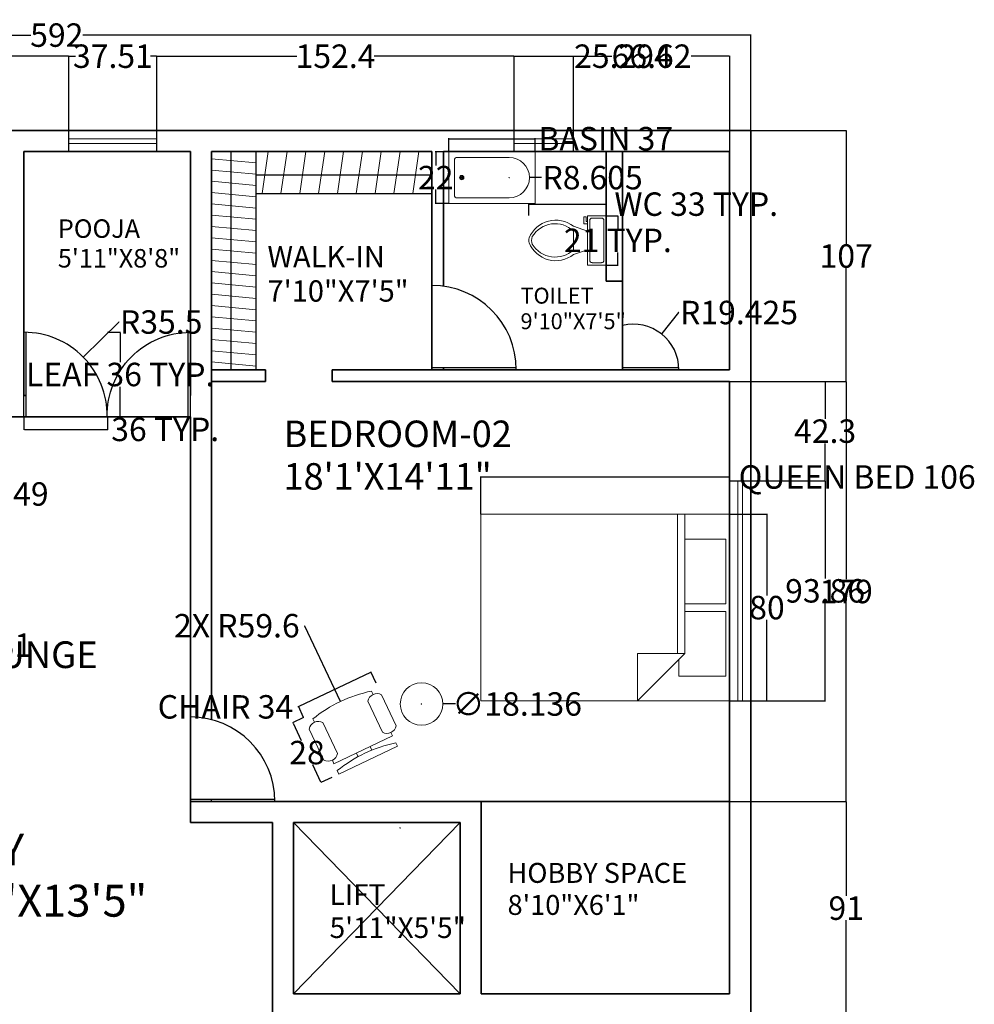
# Model space of a CAD drawing. Units: inches. Extents: x 135 to 880, y 60 to 879.
# Tile 5 of 5: x 473 to 880, y 459 to 879. Entities that reach past the tile are written whole.
import ezdxf

# ---------------------------------------------------------------- set-up
doc = ezdxf.new("R2010")
doc.units = ezdxf.units.IN
doc.header["$MEASUREMENT"] = 0
for name, color, linetype, lineweight in [('A-ANNO-DIMS', 2, 'Continuous', 18), ('A-AREA-IDEN', 7, 'Continuous', 18), ('A-DOOR', 3, 'Continuous', 25), ('A-FLOR-CASE', 32, 'Continuous', 25), ('A-FLOR-CASE-PATT', 252, 'Continuous', 13), ('A-FLOR-FIXT', 9, 'Continuous', 20), ('A-FLOR-OPEN', 8, 'Continuous', 18), ('A-FURN', 8, 'Continuous', 18), ('A-GLAZ', 4, 'Continuous', 18), ('A-WALL', 7, 'Continuous', 35)]:
    doc.layers.add(name, color=color, linetype=linetype, lineweight=lineweight)
doc.styles.get("Standard").update_dxf_attribs({"font": 'arial.ttf'})
doc.dimstyles.get("Standard").update_dxf_attribs({"dimtxt": 10, "dimasz": 0.18, "dimexe": 0.18, "dimexo": 0.0625, "dimgap": 0.09, "dimtad": 0, "dimtih": 1, "dimtoh": 1, "dimdec": 0, "dimzin": 0, "dimdsep": 46, "dimlunit": 3, "dimtxsty": 'Standard', "dimcen": 0.09, "dimadec": 0, "dimazin": 0, "dimtfac": 1, "dimtdec": 0, "dimtofl": 0, "dimtmove": 0, "dimatfit": 3, "dimfxl": 1, "dimtolj": 1, "dimtzin": 0, "dimarcsym": 0})

# ---------------------------------------------------------------- blocks, each defined once
blk = doc.blocks.new('Toilet - top')
for p, q in [((9.5, -6), (9.5, -2)), ((-8, -8.5), (-8, -8)), ((-7, -8), (-7, -9.5)), ((-4, -8), (-6, -14)), ((4, -8), (6, -14)), ((-10, -8.5), (-8, -8.5)), ((-10, -9.5), (-10, -8.5)), ((-7, -9.5), (-10, -9.5)), ((4, -14), (-4, -14))]:
    blk.add_line(p, q)
blk.add_lwpolyline([(10.5, -8), (10.5, 0), (-10.5, 0), (-10.5, -8)], close=True)
for points in [[(-9.5, -2), (-9.5, -6)], [(8.5, -1), (-8.5, -1)], [(-8.5, -7), (8.5, -7)]]:
    blk.add_lwpolyline(points)
for centre, radius, start, end in [((-8.62, -1.88), 0.884, 81.8699, 188.1301), ((8.62, -1.88), 0.884, 351.8699, 98.1301), ((-8.62, -6.12), 0.884, 171.8699, 278.1301), ((8.62, -6.12), 0.884, 261.8699, 8.1301), ((3.52, -21.58), 12.17, 141.4691, 247.9714), ((4.2, -21.82), 11.33, 136.3677, 238.9468), ((-3.52, -21.58), 12.17, 292.0284, 38.5307), ((-4.2, -21.82), 11.33, 301.053, 43.6321), ((0, -27.88), 4, 245.7318, 294.2682), ((0, -29), 4, 254.8605, 285.1395)]:
    blk.add_arc(centre, radius, start, end)
blk = doc.blocks.new('Bath Tub - 26 x 60 in.')
for p, q in [((8, -18), (10, -18)), ((9, -17), (9, -19))]:
    blk.add_line(p, q)
blk.add_lwpolyline([(0, -36), (0, 0), (60, 0), (60, -36)], close=True)
for points in [[(4, -30), (4, -6)], [(6, -4), (42, -4)], [(42, -32), (6, -32)]]:
    blk.add_lwpolyline(points)
for radius in [1.5, 1]:
    blk.add_circle((9, -18), radius)
for centre, radius, start, end in [((5.75, -5.75), 1.77, 81.8699, 188.1301), ((42, -18), 14, 270, 90), ((5.75, -30.25), 1.77, 171.8699, 278.1301)]:
    blk.add_arc(centre, radius, start, end)
blk = doc.blocks.new('Bed - Queen')
for p, q in [((0, -80.00003), (0, 0)), ((0, 0), (59.99999, 0)), ((59.99999, 0), (59.99999, -80.00003)), ((7.99999, -1.2), (28.79998, -1.2)), ((7.99999, -14.4), (7.99999, -1.2)), ((28.79998, -1.2), (28.79998, -14.4)), ((31.19999, -1.2), (51.99999, -1.2)), ((31.19999, -14.4), (31.19999, -1.2)), ((51.99999, -1.2), (51.99999, -16.4)), ((0, -14.4), (44.8, -14.4)), ((59.99999, -29.6), (44.8, -14.4)), ((44.8, -14.4), (44.8, -29.6)), ((44.8, -16.8), (0, -16.8)), ((51.99999, -16.4), (46.79936, -16.4)), ((44.8, -29.6), (59.99999, -29.6)), ((59.99999, -80.00003), (0, -80.00003))]:
    blk.add_line(p, q)
blk = doc.blocks.new('Chair - Desk')
for p, q in [((-8.5, 0), (-8.5, -1)), ((-8.5, 0), (8.5, 0)), ((8.5, 0), (8.5, -1)), ((-2, -3), (-2, -1.9355)), ((2, -1.9576), (2, -3)), ((-10.5, -5), (-10.5, -14)), ((-8.5, -3), (-8.5, -4)), ((-8.5, -3), (8.5, -3)), ((-6.5, -14), (-6.5, -5)), ((6.5, -5), (6.5, -14)), ((8.5, -3), (8.5, -4)), ((10.5, -14), (10.5, -5)), ((-8.5, -15), (-8.5, -16)), ((8.5, -15), (8.5, -16))]:
    blk.add_line(p, q)
for centre, radius, start, end in [((0, 34.625), 36.625, 256.5803, 283.4197), ((-8.5, -6.5), 2.5, 36.8699, 143.1301), ((8.5, -6.5), 2.5, 36.8699, 143.1301), ((-8.5, -12.5), 2.5, 216.8699, 323.1301), ((8.5, -12.5), 2.5, 216.8699, 323.1301), ((0, 19.625), 36.625, 256.5803, 283.4197)]:
    blk.add_arc(centre, radius, start, end)
blk = doc.blocks.new('DOOR-SWING-36IN')
for p, q in [((36, 36), (0, 36)), ((36, 35), (0, 35))]:
    blk.add_line(p, q)
blk.add_arc((36, 36), 36, 180, 270)
blk = doc.blocks.new('DOOR-PAIRED-LEAF-36IN')
for p, q in [((0, 0), (0, 36)), ((1, 0), (1, 36))]:
    blk.add_line(p, q)
blk.add_arc((0, 0.5), 35.5, 359.1987, 90)
blk = doc.blocks.new('*D12')
at = {"layer": 'A-ANNO-DIMS', "color": 0, "lineweight": -2, "transparency": 16777216}
for p, q in [((402.69, 638.57), (399.13, 635.46)), ((399.38, 635.45), (419.31, 612.59)), ((422.85, 615.44), (419.29, 612.34)), ((419.42, 612.45), (419.54, 612.32)), ((419.54, 612.32), (419.72, 612.32))]:
    blk.add_line(p, q, dxfattribs=at)
at = {"layer": 'A-ANNO-DIMS', "color": 0, "transparency": 16777216}
for points in [[(399.41, 635.47), (399.36, 635.43), (399.27, 635.58)], [(419.33, 612.61), (419.28, 612.57), (419.42, 612.45)]]:
    blk.add_solid(points, dxfattribs=at)
at = {"layer": 'Defpoints', "color": 0, "transparency": 16777216}
for p in [(402.73, 638.61), (422.89, 615.48), (419.42, 612.45)]:
    blk.add_point(p, dxfattribs=at)
at = {"layer": 'A-ANNO-DIMS', "color": 0, "transparency": 16777216, "insert": (449.62, 612.32), "char_height": 10, "attachment_point": 5}
blk.add_mtext('\\A1;CHAIR 31', dxfattribs=at)
blk = doc.blocks.new('*D16')
at = {"layer": 'A-ANNO-DIMS', "color": 0, "lineweight": -2, "transparency": 16777216}
for p, q in [((622.81, 600.64), (592.25, 586.17)), ((625.14, 596.14), (622.89, 600.88)), ((591.93, 586.01), (591.75, 586.01)), ((592.09, 586.09), (591.93, 586.01)), ((594.26, 581.51), (592.01, 586.25))]:
    blk.add_line(p, q, dxfattribs=at)
at = {"layer": 'A-ANNO-DIMS', "color": 0, "transparency": 16777216}
for points in [[(622.8, 600.67), (622.82, 600.61), (622.97, 600.72)], [(592.24, 586.19), (592.26, 586.14), (592.09, 586.09)]]:
    blk.add_solid(points, dxfattribs=at)
at = {"layer": 'Defpoints', "color": 0, "transparency": 16777216}
for p in [(625.17, 596.09), (592.09, 586.09), (594.28, 581.46)]:
    blk.add_point(p, dxfattribs=at)
at = {"layer": 'A-ANNO-DIMS', "color": 0, "transparency": 16777216, "insert": (560.9, 586.01), "char_height": 10, "attachment_point": 5}
blk.add_mtext('\\A1;CHAIR 34', dxfattribs=at)
blk = doc.blocks.new('*D17')
at = {"layer": 'A-ANNO-DIMS', "color": 0, "lineweight": -2, "transparency": 16777216}
for p, q in [((594.23, 581.43), (589.49, 579.19)), ((589.73, 579.1), (593.23, 571.71)), ((601.65, 553.94), (598.15, 561.32)), ((606.3, 555.94), (601.56, 553.7))]:
    blk.add_line(p, q, dxfattribs=at)
at = {"layer": 'A-ANNO-DIMS', "color": 0, "transparency": 16777216}
for points in [[(589.76, 579.11), (589.7, 579.09), (589.65, 579.26)], [(601.68, 553.95), (601.62, 553.92), (601.73, 553.77)]]:
    blk.add_solid(points, dxfattribs=at)
at = {"layer": 'Defpoints', "color": 0, "transparency": 16777216}
for p in [(594.28, 581.46), (606.36, 555.97), (601.73, 553.77)]:
    blk.add_point(p, dxfattribs=at)
at = {"layer": 'A-ANNO-DIMS', "color": 0, "transparency": 16777216, "insert": (595.69, 566.52), "char_height": 10, "attachment_point": 5}
blk.add_mtext('\\A1;28', dxfattribs=at)
blk = doc.blocks.new('*D20')
at = {"layer": 'A-ANNO-DIMS', "color": 0, "lineweight": -2, "transparency": 16777216}
for p, q in [((656.14, 822.76), (656.14, 828.41)), ((656.32, 828.23), (692.84, 828.23)), ((693.02, 822.76), (693.02, 828.41)), ((693.02, 828.23), (693.2, 828.23))]:
    blk.add_line(p, q, dxfattribs=at)
at = {"layer": 'A-ANNO-DIMS', "color": 0, "transparency": 16777216}
for points in [[(656.32, 828.26), (656.32, 828.2), (656.14, 828.23)], [(692.84, 828.26), (692.84, 828.2), (693.02, 828.23)]]:
    blk.add_solid(points, dxfattribs=at)
at = {"layer": 'Defpoints', "color": 0, "transparency": 16777216}
for p in [(693.02, 828.23), (656.14, 822.7), (693.02, 822.7)]:
    blk.add_point(p, dxfattribs=at)
at = {"layer": 'A-ANNO-DIMS', "color": 0, "transparency": 16777216, "insert": (723.13, 828.23), "char_height": 10, "attachment_point": 5}
blk.add_mtext('\\A1;BASIN 37', dxfattribs=at)
blk = doc.blocks.new('*D21')
at = {"layer": 'A-ANNO-DIMS', "color": 0, "lineweight": -2, "transparency": 16777216}
for p, q in [((656.08, 822.7), (650.43, 822.7)), ((650.61, 822.52), (650.61, 816.75)), ((650.61, 800.75), (650.61, 806.53)), ((656.08, 800.57), (650.43, 800.57))]:
    blk.add_line(p, q, dxfattribs=at)
at = {"layer": 'A-ANNO-DIMS', "color": 0, "transparency": 16777216}
for points in [[(650.58, 822.52), (650.64, 822.52), (650.61, 822.7)], [(650.58, 800.75), (650.64, 800.75), (650.61, 800.57)]]:
    blk.add_solid(points, dxfattribs=at)
at = {"layer": 'Defpoints', "color": 0, "transparency": 16777216}
for p in [(650.61, 822.7), (656.14, 822.7), (656.14, 800.57)]:
    blk.add_point(p, dxfattribs=at)
at = {"layer": 'A-ANNO-DIMS', "color": 0, "transparency": 16777216, "insert": (650.61, 811.64), "char_height": 10, "attachment_point": 5}
blk.add_mtext('\\A1;22', dxfattribs=at)
blk = doc.blocks.new('*D28')
at = {"layer": 'A-ANNO-DIMS', "color": 0, "lineweight": -2, "transparency": 16777216}
for p, q in [((669.88, 668.17), (669.88, 684.2)), ((670.06, 684.02), (775.8, 684.02)), ((775.98, 668.17), (775.98, 684.2)), ((775.98, 684.02), (776.16, 684.02))]:
    blk.add_line(p, q, dxfattribs=at)
at = {"layer": 'A-ANNO-DIMS', "color": 0, "transparency": 16777216}
for points in [[(670.06, 684.05), (670.06, 683.99), (669.88, 684.02)], [(775.8, 684.05), (775.8, 683.99), (775.98, 684.02)]]:
    blk.add_solid(points, dxfattribs=at)
at = {"layer": 'Defpoints', "color": 0, "transparency": 16777216}
for p in [(775.98, 684.02), (669.88, 668.1), (775.98, 668.1)]:
    blk.add_point(p, dxfattribs=at)
at = {"layer": 'A-ANNO-DIMS', "color": 0, "transparency": 16777216, "insert": (830.36, 684.02), "char_height": 10, "attachment_point": 5}
blk.add_mtext('\\A1;QUEEN BED 106', dxfattribs=at)
blk = doc.blocks.new('*D29')
at = {"layer": 'A-ANNO-DIMS', "color": 0, "lineweight": -2, "transparency": 16777216}
for p, q in [((776.04, 668.1), (792.07, 668.1)), ((791.89, 667.92), (791.89, 633.52)), ((791.89, 588.72), (791.89, 623.12)), ((776.04, 588.54), (792.07, 588.54))]:
    blk.add_line(p, q, dxfattribs=at)
at = {"layer": 'A-ANNO-DIMS', "color": 0, "transparency": 16777216}
for points in [[(791.86, 667.92), (791.92, 667.92), (791.89, 668.1)], [(791.86, 588.72), (791.92, 588.72), (791.89, 588.54)]]:
    blk.add_solid(points, dxfattribs=at)
at = {"layer": 'Defpoints', "color": 0, "transparency": 16777216}
for p in [(775.98, 668.1), (775.98, 588.54), (791.89, 588.54)]:
    blk.add_point(p, dxfattribs=at)
at = {"layer": 'A-ANNO-DIMS', "color": 0, "transparency": 16777216, "insert": (791.89, 628.32), "char_height": 10, "attachment_point": 5}
blk.add_mtext('\\A1;80', dxfattribs=at)
blk = doc.blocks.new('*D30')
at = {"layer": 'A-ANNO-DIMS', "color": 0, "lineweight": -2, "transparency": 16777216}
for p, q in [((690.28, 795.44), (690.28, 800.51)), ((690.46, 800.33), (723.15, 800.33)), ((723.33, 795.44), (723.33, 800.51)), ((723.33, 800.33), (723.51, 800.33))]:
    blk.add_line(p, q, dxfattribs=at)
at = {"layer": 'A-ANNO-DIMS', "color": 0, "transparency": 16777216}
for points in [[(690.46, 800.36), (690.46, 800.3), (690.28, 800.33)], [(723.15, 800.36), (723.15, 800.3), (723.33, 800.33)]]:
    blk.add_solid(points, dxfattribs=at)
at = {"layer": 'Defpoints', "color": 0, "transparency": 16777216}
for p in [(723.33, 800.33), (690.28, 795.38), (723.33, 795.38)]:
    blk.add_point(p, dxfattribs=at)
at = {"layer": 'A-ANNO-DIMS', "color": 0, "transparency": 16777216, "insert": (761.72, 800.33), "char_height": 10, "attachment_point": 5}
blk.add_mtext('\\A1;WC 33 TYP.', dxfattribs=at)
blk = doc.blocks.new('*D31')
at = {"layer": 'A-ANNO-DIMS', "color": 0, "lineweight": -2, "transparency": 16777216}
for p, q in [((723.39, 795.38), (728.47, 795.38)), ((728.29, 795.2), (728.29, 789.99)), ((728.29, 774.56), (728.29, 779.76)), ((723.39, 774.38), (728.47, 774.38))]:
    blk.add_line(p, q, dxfattribs=at)
at = {"layer": 'A-ANNO-DIMS', "color": 0, "transparency": 16777216}
for points in [[(728.26, 795.2), (728.32, 795.2), (728.29, 795.38)], [(728.26, 774.56), (728.32, 774.56), (728.29, 774.38)]]:
    blk.add_solid(points, dxfattribs=at)
at = {"layer": 'Defpoints', "color": 0, "transparency": 16777216}
for p in [(723.33, 795.38), (723.33, 774.38), (728.29, 774.38)]:
    blk.add_point(p, dxfattribs=at)
at = {"layer": 'A-ANNO-DIMS', "color": 0, "transparency": 16777216, "insert": (728.29, 784.88), "char_height": 10, "attachment_point": 5}
blk.add_mtext('\\A1;21 TYP.', dxfattribs=at)
blk = doc.blocks.new('*D34')
at = {"layer": 'A-ANNO-DIMS', "color": 0, "lineweight": -2, "transparency": 16777216}
for p, q in [((510.67, 745.7), (516.19, 745.7)), ((516.01, 745.52), (516.01, 732.9)), ((516.01, 709.88), (516.01, 722.5)), ((510.67, 709.7), (516.19, 709.7))]:
    blk.add_line(p, q, dxfattribs=at)
at = {"layer": 'A-ANNO-DIMS', "color": 0, "transparency": 16777216}
for points in [[(515.98, 745.52), (516.04, 745.52), (516.01, 745.7)], [(515.98, 709.88), (516.04, 709.88), (516.01, 709.7)]]:
    blk.add_solid(points, dxfattribs=at)
at = {"layer": 'Defpoints', "color": 0, "transparency": 16777216}
for p in [(510.61, 745.7), (516.01, 745.7), (510.61, 709.7)]:
    blk.add_point(p, dxfattribs=at)
at = {"layer": 'A-ANNO-DIMS', "color": 0, "transparency": 16777216, "insert": (516.01, 727.7), "char_height": 10, "attachment_point": 5}
blk.add_mtext('\\A1;LEAF 36 TYP.', dxfattribs=at)
blk = doc.blocks.new('*D35')
at = {"layer": 'A-ANNO-DIMS', "color": 0, "lineweight": -2, "transparency": 16777216}
for p, q in [((474.98, 709.64), (474.98, 704.12)), ((510.61, 709.64), (510.61, 704.12)), ((475.16, 704.3), (510.43, 704.3)), ((510.61, 704.3), (510.79, 704.3))]:
    blk.add_line(p, q, dxfattribs=at)
at = {"layer": 'A-ANNO-DIMS', "color": 0, "transparency": 16777216}
for points in [[(475.16, 704.33), (475.16, 704.27), (474.98, 704.3)], [(510.43, 704.33), (510.43, 704.27), (510.61, 704.3)]]:
    blk.add_solid(points, dxfattribs=at)
at = {"layer": 'Defpoints', "color": 0, "transparency": 16777216}
for p in [(474.98, 709.7), (510.61, 709.7), (510.61, 704.3)]:
    blk.add_point(p, dxfattribs=at)
at = {"layer": 'A-ANNO-DIMS', "color": 0, "transparency": 16777216, "insert": (535.21, 704.3), "char_height": 10, "attachment_point": 5}
blk.add_mtext('\\A1;36 TYP.', dxfattribs=at)
blk = doc.blocks.new('*D38')
at = {"layer": 'A-ANNO-DIMS', "color": 0, "lineweight": -2, "transparency": 16777216}
for p, q in [((192.98, 831.76), (192.98, 872.58)), ((193.16, 872.4), (477.89, 872.4)), ((784.8, 872.4), (500.06, 872.4)), ((784.98, 831.76), (784.98, 872.58))]:
    blk.add_line(p, q, dxfattribs=at)
at = {"layer": 'A-ANNO-DIMS', "color": 0, "transparency": 16777216}
for points in [[(193.16, 872.43), (193.16, 872.37), (192.98, 872.4)], [(784.8, 872.43), (784.8, 872.37), (784.98, 872.4)]]:
    blk.add_solid(points, dxfattribs=at)
at = {"layer": 'Defpoints', "color": 0, "transparency": 16777216}
for p in [(784.98, 872.4), (192.98, 831.7), (784.98, 831.7)]:
    blk.add_point(p, dxfattribs=at)
at = {"layer": 'A-ANNO-DIMS', "color": 0, "transparency": 16777216, "insert": (488.98, 872.4), "char_height": 10, "attachment_point": 5}
blk.add_mtext('\\A1;592', dxfattribs=at)
blk = doc.blocks.new('*D40')
at = {"layer": 'A-ANNO-DIMS', "color": 0, "lineweight": -2, "transparency": 16777216}
for p, q in [((192.98, 822.76), (192.98, 863.58)), ((193.16, 863.4), (326.65, 863.4)), ((493.97, 863.4), (360.47, 863.4)), ((494.15, 822.76), (494.15, 863.58))]:
    blk.add_line(p, q, dxfattribs=at)
at = {"layer": 'A-ANNO-DIMS', "color": 0, "transparency": 16777216}
for points in [[(193.16, 863.43), (193.16, 863.37), (192.98, 863.4)], [(493.97, 863.43), (493.97, 863.37), (494.15, 863.4)]]:
    blk.add_solid(points, dxfattribs=at)
at = {"layer": 'Defpoints', "color": 0, "transparency": 16777216}
for p in [(494.15, 863.4), (192.98, 822.7), (494.15, 822.7)]:
    blk.add_point(p, dxfattribs=at)
at = {"layer": 'A-ANNO-DIMS', "color": 0, "transparency": 16777216, "insert": (343.56, 863.4), "char_height": 10, "attachment_point": 5}
blk.add_mtext('\\A1;301.2', dxfattribs=at)
blk = doc.blocks.new('*D41')
at = {"layer": 'A-ANNO-DIMS', "color": 0, "lineweight": -2, "transparency": 16777216}
for p, q in [((494.15, 822.76), (494.15, 863.58)), ((494.33, 863.4), (496.91, 863.4)), ((531.47, 863.4), (528.89, 863.4)), ((531.65, 822.76), (531.65, 863.58))]:
    blk.add_line(p, q, dxfattribs=at)
at = {"layer": 'A-ANNO-DIMS', "color": 0, "transparency": 16777216}
for points in [[(494.33, 863.43), (494.33, 863.37), (494.15, 863.4)], [(531.47, 863.43), (531.47, 863.37), (531.65, 863.4)]]:
    blk.add_solid(points, dxfattribs=at)
at = {"layer": 'Defpoints', "color": 0, "transparency": 16777216}
for p in [(531.65, 863.4), (494.15, 822.7), (531.65, 822.7)]:
    blk.add_point(p, dxfattribs=at)
at = {"layer": 'A-ANNO-DIMS', "color": 0, "transparency": 16777216, "insert": (512.9, 863.4), "char_height": 10, "attachment_point": 5}
blk.add_mtext('\\A1;37.51', dxfattribs=at)
blk = doc.blocks.new('*D42')
at = {"layer": 'A-ANNO-DIMS', "color": 0, "lineweight": -2, "transparency": 16777216}
for p, q in [((531.65, 822.76), (531.65, 863.58)), ((531.83, 863.4), (591.38, 863.4)), ((683.88, 863.4), (624.33, 863.4)), ((684.06, 822.76), (684.06, 863.58))]:
    blk.add_line(p, q, dxfattribs=at)
at = {"layer": 'A-ANNO-DIMS', "color": 0, "transparency": 16777216}
for points in [[(531.83, 863.43), (531.83, 863.37), (531.65, 863.4)], [(683.88, 863.43), (683.88, 863.37), (684.06, 863.4)]]:
    blk.add_solid(points, dxfattribs=at)
at = {"layer": 'Defpoints', "color": 0, "transparency": 16777216}
for p in [(684.06, 863.4), (531.65, 822.7), (684.06, 822.7)]:
    blk.add_point(p, dxfattribs=at)
at = {"layer": 'A-ANNO-DIMS', "color": 0, "transparency": 16777216, "insert": (607.86, 863.4), "char_height": 10, "attachment_point": 5}
blk.add_mtext('\\A1;152.4', dxfattribs=at)
blk = doc.blocks.new('*D43')
at = {"layer": 'A-ANNO-DIMS', "color": 0, "lineweight": -2, "transparency": 16777216}
for p, q in [((684.06, 822.76), (684.06, 863.58)), ((684.24, 863.4), (709.17, 863.4)), ((709.35, 822.76), (709.35, 863.58)), ((709.35, 863.4), (709.53, 863.4))]:
    blk.add_line(p, q, dxfattribs=at)
at = {"layer": 'A-ANNO-DIMS', "color": 0, "transparency": 16777216}
for points in [[(684.24, 863.43), (684.24, 863.37), (684.06, 863.4)], [(709.17, 863.43), (709.17, 863.37), (709.35, 863.4)]]:
    blk.add_solid(points, dxfattribs=at)
at = {"layer": 'Defpoints', "color": 0, "transparency": 16777216}
for p in [(709.35, 863.4), (684.06, 822.7), (709.35, 822.7)]:
    blk.add_point(p, dxfattribs=at)
at = {"layer": 'A-ANNO-DIMS', "color": 0, "transparency": 16777216, "insert": (730.44, 863.4), "char_height": 10, "attachment_point": 5}
blk.add_mtext('\\A1;25.294', dxfattribs=at)
blk = doc.blocks.new('*D44')
at = {"layer": 'A-ANNO-DIMS', "color": 0, "lineweight": -2, "transparency": 16777216}
for p, q in [((709.35, 822.76), (709.35, 863.58)), ((709.53, 863.4), (725.73, 863.4)), ((775.8, 863.4), (759.6, 863.4)), ((775.98, 822.76), (775.98, 863.58))]:
    blk.add_line(p, q, dxfattribs=at)
at = {"layer": 'A-ANNO-DIMS', "color": 0, "transparency": 16777216}
for points in [[(709.53, 863.43), (709.53, 863.37), (709.35, 863.4)], [(775.8, 863.43), (775.8, 863.37), (775.98, 863.4)]]:
    blk.add_solid(points, dxfattribs=at)
at = {"layer": 'Defpoints', "color": 0, "transparency": 16777216}
for p in [(775.98, 863.4), (709.35, 822.7), (775.98, 822.7)]:
    blk.add_point(p, dxfattribs=at)
at = {"layer": 'A-ANNO-DIMS', "color": 0, "transparency": 16777216, "insert": (742.66, 863.4), "char_height": 10, "attachment_point": 5}
blk.add_mtext('\\A1;66.62', dxfattribs=at)
blk = doc.blocks.new('*D63')
at = {"layer": 'A-ANNO-DIMS', "color": 0, "lineweight": -2, "transparency": 16777216}
for p, q in [((776.04, 545.7), (825.86, 545.7)), ((825.68, 545.52), (825.68, 505.4)), ((825.68, 454.88), (825.68, 495.01)), ((785.04, 454.7), (825.86, 454.7))]:
    blk.add_line(p, q, dxfattribs=at)
at = {"layer": 'A-ANNO-DIMS', "color": 0, "transparency": 16777216}
for points in [[(825.65, 545.52), (825.71, 545.52), (825.68, 545.7)], [(825.65, 454.88), (825.71, 454.88), (825.68, 454.7)]]:
    blk.add_solid(points, dxfattribs=at)
at = {"layer": 'Defpoints', "color": 0, "transparency": 16777216}
for p in [(775.98, 545.7), (825.68, 545.7), (784.98, 454.7)]:
    blk.add_point(p, dxfattribs=at)
at = {"layer": 'A-ANNO-DIMS', "color": 0, "transparency": 16777216, "insert": (825.68, 500.2), "char_height": 10, "attachment_point": 5}
blk.add_mtext('\\A1;91', dxfattribs=at)
blk = doc.blocks.new('*D64')
at = {"layer": 'A-ANNO-DIMS', "color": 0, "lineweight": -2, "transparency": 16777216}
for p, q in [((776.04, 724.7), (825.86, 724.7)), ((825.68, 724.52), (825.68, 640.4)), ((825.68, 545.88), (825.68, 630.01)), ((776.04, 545.7), (825.86, 545.7))]:
    blk.add_line(p, q, dxfattribs=at)
at = {"layer": 'A-ANNO-DIMS', "color": 0, "transparency": 16777216}
for points in [[(825.65, 724.52), (825.71, 724.52), (825.68, 724.7)], [(825.65, 545.88), (825.71, 545.88), (825.68, 545.7)]]:
    blk.add_solid(points, dxfattribs=at)
at = {"layer": 'Defpoints', "color": 0, "transparency": 16777216}
for p in [(775.98, 724.7), (825.68, 724.7), (775.98, 545.7)]:
    blk.add_point(p, dxfattribs=at)
at = {"layer": 'A-ANNO-DIMS', "color": 0, "transparency": 16777216, "insert": (825.68, 635.2), "char_height": 10, "attachment_point": 5}
blk.add_mtext('\\A1;179', dxfattribs=at)
blk = doc.blocks.new('*D65')
at = {"layer": 'A-ANNO-DIMS', "color": 0, "lineweight": -2, "transparency": 16777216}
for p, q in [((785.04, 831.7), (825.86, 831.7)), ((825.68, 831.52), (825.68, 783.4)), ((825.68, 724.88), (825.68, 773.01)), ((776.04, 724.7), (825.86, 724.7))]:
    blk.add_line(p, q, dxfattribs=at)
at = {"layer": 'A-ANNO-DIMS', "color": 0, "transparency": 16777216}
for points in [[(825.65, 831.52), (825.71, 831.52), (825.68, 831.7)], [(825.65, 724.88), (825.71, 724.88), (825.68, 724.7)]]:
    blk.add_solid(points, dxfattribs=at)
at = {"layer": 'Defpoints', "color": 0, "transparency": 16777216}
for p in [(784.98, 831.7), (825.68, 831.7), (775.98, 724.7)]:
    blk.add_point(p, dxfattribs=at)
at = {"layer": 'A-ANNO-DIMS', "color": 0, "transparency": 16777216, "insert": (825.68, 778.2), "char_height": 10, "attachment_point": 5}
blk.add_mtext('\\A1;107', dxfattribs=at)
blk = doc.blocks.new('*D70')
at = {"layer": 'A-ANNO-DIMS', "color": 0, "lineweight": -2, "transparency": 16777216}
for p, q in [((776.04, 724.7), (816.86, 724.7)), ((816.68, 724.52), (816.68, 708.75)), ((816.68, 682.58), (816.68, 698.35)), ((776.04, 682.4), (816.86, 682.4))]:
    blk.add_line(p, q, dxfattribs=at)
at = {"layer": 'A-ANNO-DIMS', "color": 0, "transparency": 16777216}
for points in [[(816.65, 724.52), (816.71, 724.52), (816.68, 724.7)], [(816.65, 682.58), (816.71, 682.58), (816.68, 682.4)]]:
    blk.add_solid(points, dxfattribs=at)
at = {"layer": 'Defpoints', "color": 0, "transparency": 16777216}
for p in [(775.98, 724.7), (775.98, 682.4), (816.68, 682.4)]:
    blk.add_point(p, dxfattribs=at)
at = {"layer": 'A-ANNO-DIMS', "color": 0, "transparency": 16777216, "insert": (816.68, 703.55), "char_height": 10, "attachment_point": 5}
blk.add_mtext('\\A1;42.3', dxfattribs=at)
blk = doc.blocks.new('*D71')
at = {"layer": 'A-ANNO-DIMS', "color": 0, "lineweight": -2, "transparency": 16777216}
for p, q in [((776.04, 682.4), (816.86, 682.4)), ((816.68, 682.22), (816.68, 640.67)), ((816.68, 588.72), (816.68, 630.27)), ((776.04, 588.54), (816.86, 588.54))]:
    blk.add_line(p, q, dxfattribs=at)
at = {"layer": 'A-ANNO-DIMS', "color": 0, "transparency": 16777216}
for points in [[(816.65, 682.22), (816.71, 682.22), (816.68, 682.4)], [(816.65, 588.72), (816.71, 588.72), (816.68, 588.54)]]:
    blk.add_solid(points, dxfattribs=at)
at = {"layer": 'Defpoints', "color": 0, "transparency": 16777216}
for p in [(775.98, 682.4), (775.98, 588.54), (816.68, 588.54)]:
    blk.add_point(p, dxfattribs=at)
at = {"layer": 'A-ANNO-DIMS', "color": 0, "transparency": 16777216, "insert": (816.68, 635.47), "char_height": 10, "attachment_point": 5}
blk.add_mtext('\\A1;93.86', dxfattribs=at)
blk = doc.blocks.new('*D76')
at = {"layer": 'A-ANNO-DIMS', "color": 0, "lineweight": -2, "transparency": 16777216}
for p, q in [((754.12, 754.13), (747.03, 745.11)), ((754.3, 754.13), (754.12, 754.13)), ((734.82, 729.7), (735, 729.7)), ((734.91, 729.61), (734.91, 729.79))]:
    blk.add_line(p, q, dxfattribs=at)
at = {"layer": 'A-ANNO-DIMS', "color": 0, "transparency": 16777216}
blk.add_solid([(747, 745.13), (747.05, 745.09), (746.91, 744.97)], dxfattribs=at)
at = {"layer": 'Defpoints', "color": 0, "transparency": 16777216}
for p in [(746.91, 744.97), (734.91, 729.7)]:
    blk.add_point(p, dxfattribs=at)
at = {"layer": 'A-ANNO-DIMS', "color": 0, "transparency": 16777216, "insert": (779.97, 754.13), "char_height": 10, "attachment_point": 5}
blk.add_mtext('\\A1;R19.425', dxfattribs=at)
blk = doc.blocks.new('*D77')
at = {"layer": 'A-ANNO-DIMS', "color": 0, "lineweight": -2, "transparency": 16777216}
for p, q in [((515.42, 750.08), (500.38, 735.25)), ((515.6, 750.08), (515.42, 750.08)), ((474.89, 710.2), (475.07, 710.2)), ((474.98, 710.11), (474.98, 710.29))]:
    blk.add_line(p, q, dxfattribs=at)
at = {"layer": 'A-ANNO-DIMS', "color": 0, "transparency": 16777216}
blk.add_solid([(500.36, 735.27), (500.4, 735.23), (500.26, 735.13)], dxfattribs=at)
at = {"layer": 'Defpoints', "color": 0, "transparency": 16777216}
for p in [(500.26, 735.13), (474.98, 710.2)]:
    blk.add_point(p, dxfattribs=at)
at = {"layer": 'A-ANNO-DIMS', "color": 0, "transparency": 16777216, "insert": (533.5, 750.08), "char_height": 10, "attachment_point": 5}
blk.add_mtext('\\A1;R35.5', dxfattribs=at)
blk = doc.blocks.new('*D81')
at = {"layer": 'A-ANNO-DIMS', "color": 0, "lineweight": -2, "transparency": 16777216}
for p, q in [((417.13, 676.77), (417.31, 676.77)), ((417.22, 676.68), (417.22, 676.86)), ((439.22, 676.77), (431.15, 676.77))]:
    blk.add_line(p, q, dxfattribs=at)
at = {"layer": 'A-ANNO-DIMS', "color": 0, "transparency": 16777216}
blk.add_solid([(431.15, 676.8), (431.15, 676.74), (430.97, 676.77)], dxfattribs=at)
at = {"layer": 'Defpoints', "color": 0, "transparency": 16777216}
for p in [(403.48, 676.77), (430.97, 676.77)]:
    blk.add_point(p, dxfattribs=at)
at = {"layer": 'A-ANNO-DIMS', "color": 0, "transparency": 16777216, "insert": (461.63, 676.77), "char_height": 10, "attachment_point": 5}
blk.add_mtext('\\A1;∅27.49', dxfattribs=at)
blk = doc.blocks.new('*D82')
at = {"layer": 'A-ANNO-DIMS', "color": 0, "lineweight": -2, "transparency": 16777216}
for p, q in [((644.45, 587.23), (644.63, 587.23)), ((644.54, 587.14), (644.54, 587.32)), ((659.05, 587.23), (653.79, 587.23))]:
    blk.add_line(p, q, dxfattribs=at)
at = {"layer": 'A-ANNO-DIMS', "color": 0, "transparency": 16777216}
blk.add_solid([(653.79, 587.26), (653.79, 587.2), (653.61, 587.23)], dxfattribs=at)
at = {"layer": 'Defpoints', "color": 0, "transparency": 16777216}
for p in [(635.48, 587.23), (653.61, 587.23)]:
    blk.add_point(p, dxfattribs=at)
at = {"layer": 'A-ANNO-DIMS', "color": 0, "transparency": 16777216, "insert": (685.34, 587.23), "char_height": 10, "attachment_point": 5}
blk.add_mtext('\\A1;∅18.136', dxfattribs=at)
blk = doc.blocks.new('*D86')
at = {"layer": 'A-ANNO-DIMS', "color": 0, "lineweight": -2, "transparency": 16777216}
for p, q in [((594.47, 620.6), (594.65, 620.6)), ((594.65, 620.6), (609.88, 588.44)), ((635.38, 534.42), (635.56, 534.42)), ((635.47, 534.33), (635.47, 534.51))]:
    blk.add_line(p, q, dxfattribs=at)
at = {"layer": 'A-ANNO-DIMS', "color": 0, "transparency": 16777216}
blk.add_solid([(609.91, 588.46), (609.85, 588.43), (609.96, 588.28)], dxfattribs=at)
at = {"layer": 'Defpoints', "color": 0, "transparency": 16777216}
for p in [(609.96, 588.28), (635.47, 534.42)]:
    blk.add_point(p, dxfattribs=at)
at = {"layer": 'A-ANNO-DIMS', "color": 0, "transparency": 16777216, "insert": (565.78, 620.6), "char_height": 10, "attachment_point": 5}
blk.add_mtext('\\A1;2X R59.6', dxfattribs=at)
blk = doc.blocks.new('*D92')
at = {"layer": 'A-ANNO-DIMS', "color": 0, "lineweight": -2, "transparency": 16777216}
for p, q in [((681.87, 811.64), (682.05, 811.64)), ((681.96, 811.55), (681.96, 811.73)), ((695.72, 811.64), (690.74, 811.64))]:
    blk.add_line(p, q, dxfattribs=at)
at = {"layer": 'A-ANNO-DIMS', "color": 0, "transparency": 16777216}
blk.add_solid([(690.74, 811.67), (690.74, 811.61), (690.56, 811.64)], dxfattribs=at)
at = {"layer": 'Defpoints', "color": 0, "transparency": 16777216}
for p in [(681.96, 811.64), (690.56, 811.64)]:
    blk.add_point(p, dxfattribs=at)
at = {"layer": 'A-ANNO-DIMS', "color": 0, "transparency": 16777216, "insert": (717.51, 811.64), "char_height": 10, "attachment_point": 5}
blk.add_mtext('\\A1;R8.605', dxfattribs=at)

msp = doc.modelspace()

# ---------------------------------------------------------------- hatches: boundary and pattern name
at = {"layer": 'A-FLOR-CASE-PATT'}
h = msp.add_hatch(dxfattribs=at)
h.set_pattern_fill('ANSI31', color=256, scale=38.34918, angle=129.6758, style=0)
h.paths.add_polyline_path([(567.4528, 729.7014), (573.9538, 729.7014), (573.9538, 820.0881), (554.9753, 821.8567), (554.9753, 730.8642)])
h = msp.add_hatch(dxfattribs=at)
h.set_pattern_fill('ANSI31', color=256, scale=63.5704, angle=36.6119, style=0)
h.paths.add_polyline_path([(573.9538, 804.8555), (644.3894, 804.8555), (647.0209, 822.7014), (575.5341, 822.7014), (573.9538, 811.9846)])

# ---------------------------------------------------------------- linework, layer by layer
at = {"layer": 'A-DOOR'}
for p, q in [((653.9753, 765.3525), (653.9753, 765.7014)), ((648.9753, 730.7014), (648.9753, 729.7014)), ((653.9753, 729.7014), (653.9753, 730.7014)), ((653.9753, 730.7014), (653.9753, 729.7014)), ((730.3302, 730.7014), (754.3302, 730.7014)), ((648.9753, 729.7014), (684.9753, 729.7014)), ((653.9753, 729.7014), (689.9753, 729.7014)), ((730.3302, 729.7014), (754.3302, 729.7014)), ((474.9753, 718.7014), (475.9753, 718.7014)), ((475.9753, 718.7014), (474.9753, 718.7014)), ((554.9753, 545.7014), (554.9753, 546.7014))]:
    msp.add_line(p, q, dxfattribs=at)
msp.add_arc((734.905, 729.7014), 19.4252, 0, 103.621641, dxfattribs=at)
at = {"layer": 'A-FLOR-CASE'}
for p, q in [((563.2995, 729.7014), (563.2995, 822.7014)), ((573.9538, 729.7014), (573.9538, 822.7014)), ((573.9538, 812.8858), (648.9753, 812.8858)), ((573.9538, 804.8555), (648.9753, 804.8555))]:
    msp.add_line(p, q, dxfattribs=at)
at = {"layer": 'A-FLOR-OPEN'}
for p, q in [((589.9753, 536.7014), (660.9753, 463.7014)), ((589.9753, 463.7014), (660.9753, 536.7014))]:
    msp.add_line(p, q, dxfattribs=at)
at = {"layer": 'A-FURN'}
msp.add_circle((644.5435, 587.227), 9.0679, dxfattribs=at)
at = {"layer": 'A-GLAZ'}
for p, q in [((494.1454, 831.7014), (494.1454, 822.7014)), ((531.6524, 831.7014), (531.6524, 822.7014)), ((684.0582, 831.7014), (684.0582, 822.7014)), ((709.3518, 831.7014), (709.3518, 822.7014)), ((494.1454, 828.2014), (531.6524, 828.2014)), ((684.0582, 828.2014), (709.3518, 828.2014)), ((494.1454, 826.2014), (531.6524, 826.2014)), ((684.0582, 826.2014), (709.3518, 826.2014)), ((775.9753, 682.4008), (784.9753, 682.4008)), ((779.4753, 682.4008), (779.4753, 588.5362)), ((781.4753, 682.4008), (781.4753, 588.5362)), ((775.9753, 588.5362), (784.9753, 588.5362))]:
    msp.add_line(p, q, dxfattribs=at)
at = {"layer": 'A-WALL'}
for p, q in [((474.9753, 831.7014), (269.9753, 831.7014)), ((474.9753, 831.7014), (554.9753, 831.7014)), ((554.9753, 831.7014), (657.9753, 831.7014)), ((657.9753, 831.7014), (784.9753, 831.7014)), ((784.9753, 831.7014), (784.9753, 724.7014)), ((474.9753, 822.7014), (545.9753, 822.7014)), ((474.9753, 718.7014), (474.9753, 822.7014)), ((545.9753, 822.7014), (545.9753, 718.7014)), ((554.9753, 822.7014), (554.9753, 733.7014)), ((554.9753, 822.7014), (648.9753, 822.7014)), ((648.9753, 822.7014), (648.9753, 729.7014)), ((653.9753, 822.7014), (775.9753, 822.7014)), ((653.9753, 822.7014), (653.9753, 765.3525)), ((723.3302, 767.459), (723.3302, 822.7014)), ((730.3302, 822.7014), (730.3302, 767.459)), ((775.9753, 822.7014), (775.9753, 729.7014)), ((730.3302, 767.459), (723.3302, 767.459)), ((723.3302, 767.459), (723.3302, 767.459)), ((730.3302, 767.459), (730.3302, 729.7014)), ((554.9753, 733.7014), (554.9753, 709.7014)), ((578.0221, 729.7014), (554.9753, 729.7014)), ((578.0221, 729.7014), (578.0221, 724.7014)), ((648.9753, 729.7014), (606.4753, 729.7014)), ((606.4753, 729.7014), (606.4753, 724.7014)), ((775.9753, 729.7014), (648.9753, 729.7014)), ((578.0221, 724.7014), (554.9753, 724.7014)), ((657.9753, 724.7014), (606.4753, 724.7014)), ((775.9753, 724.7014), (657.9753, 724.7014)), ((775.9753, 724.7014), (775.9753, 545.7014)), ((784.9753, 724.7014), (784.9753, 536.7014)), ((474.9753, 709.7014), (269.9753, 709.7014)), ((545.9753, 709.7014), (474.9753, 709.7014)), ((545.9753, 536.7014), (545.9753, 709.7014)), ((554.9753, 580.5582), (554.9753, 709.7014)), ((775.9753, 588.5362), (775.9753, 463.7014)), ((669.9753, 545.7014), (545.9753, 545.7014)), ((669.9753, 463.7014), (669.9753, 545.7014)), ((669.9753, 545.7014), (775.9753, 545.7014)), ((580.9753, 536.7014), (545.9753, 536.7014)), ((580.9753, 454.7014), (580.9753, 536.7014)), ((589.9753, 463.7014), (589.9753, 536.7014)), ((660.9753, 536.7014), (589.9753, 536.7014)), ((660.9753, 463.7014), (660.9753, 536.7014)), ((784.9753, 536.7014), (784.9753, 454.7014)), ((660.9753, 463.7014), (589.9753, 463.7014)), ((775.9753, 463.7014), (669.9753, 463.7014))]:
    msp.add_line(p, q, dxfattribs=at)

# ---------------------------------------------------------------- block references
at = {"layer": 'A-DOOR', "rotation": 180}
for p in [(684.9756, 765.7018), (581.9756, 581.7018)]:
    msp.add_blockref('DOOR-SWING-36IN', p, dxfattribs=at)
at = {"layer": 'A-DOOR'}
msp.add_blockref('DOOR-PAIRED-LEAF-36IN', (474.975, 709.701), dxfattribs=at)
at = {"layer": 'A-DOOR', "extrusion": (0, 0, -1), "zscale": -1}
msp.add_blockref('DOOR-PAIRED-LEAF-36IN', (-545.9756, 709.701), dxfattribs=at)
at = {"layer": 'A-FLOR-FIXT', "xscale": 0.6146362971528592, "yscale": 0.6146362971528592, "zscale": 0.6146362971528592}
msp.add_blockref('Bath Tub - 26 x 60 in.', (656.1413, 822.7014), dxfattribs=at)
at = {"layer": 'A-FLOR-FIXT', "rotation": 270}
msp.add_blockref('Toilet - top', (723.3302, 784.8772), dxfattribs=at)
at = {"layer": 'A-FURN'}
for name, p, xscale, yscale, zscale, rotation in [('Bed - Queen', (775.9753, 668.105), 1.326146577815825, 1.326146577815825, 1.326146577815825, 269.9999999999999), ('Chair - Desk', (621.7986, 563.2815), 1.627225619438762, 1.627225619438762, 1.627225619438762, 205.3461759419465)]:
    msp.add_blockref(name, p, dxfattribs=dict(at, xscale=xscale, yscale=yscale, zscale=zscale, rotation=rotation))

# ---------------------------------------------------------------- texts
at = {"layer": 'A-AREA-IDEN'}
for s, height, p in [('POOJA  ', 7.87984, (489.4301, 785.9634)), ('5\'11"X8\'8"', 7.87984, (489.4301, 773.3052)), ('WALK-IN', 9.09203, (578.832, 773.3649)), ('7\'10"X7\'5"', 9.09203, (578.832, 758.7594)), ('TOILET', 6.78817, (686.7645, 757.9136)), ('9\'10"X7\'5"', 6.78817, (686.7645, 747.009)), ('BEDROOM-02', 11.28812, (585.6846, 696.7674)), ('18\'1\'X14\'11"', 11.28812, (585.6846, 678.634)), ('FAMILY LOUNGE ', 11.388789, (388.8064, 602.5497)), ('LOBBY', 13.59119, (417.0166, 518.4017)), ('HOBBY SPACE ', 8.497913, (681.2301, 510.9774)), ('11\'10"X13\'5"', 13.591192, (417.0166, 496.5687)), ('LIFT', 8.78955, (605.3332, 501.5862)), ('8\'10"X6\'1"', 8.49791, (681.2301, 497.3262)), ('5\'11"X5\'5"', 8.78955, (605.3332, 487.4665))]:
    msp.add_text(s, height=height, dxfattribs=at).set_placement(p)

# ---------------------------------------------------------------- dimensions: what is measured, and where the dimension line sits
at = {"layer": 'A-ANNO-DIMS'}
for base, p1, p2, override, picture, middle in [((784.9753, 872.4014), (192.9753, 831.7014), (784.9753, 831.7014), {"dimdec": 0, "dimlfac": 1, "dimrnd": 0, "dimzin": 0, "dimdsep": 46, "dimlunit": 2}, '*D38', (488.9753, 872.4014)), ((494.1454, 863.4014), (192.9753, 822.7014), (494.1454, 822.7014), {"dimdec": 1, "dimlfac": 1, "dimrnd": 0, "dimzin": 0, "dimdsep": 46, "dimlunit": 2}, '*D40', (343.5604, 863.4014)), ((531.6524, 863.4014), (494.1454, 822.7014), (531.6524, 822.7014), {"dimdec": 2, "dimlfac": 1, "dimrnd": 0, "dimzin": 0, "dimdsep": 46, "dimlunit": 2}, '*D41', (512.8989, 863.4014)), ((684.0582, 863.4014), (531.6524, 822.7014), (684.0582, 822.7014), {"dimdec": 1, "dimlfac": 1, "dimrnd": 0, "dimzin": 0, "dimdsep": 46, "dimlunit": 2}, '*D42', (607.8553, 863.4014)), ((709.3518, 863.4014), (684.0582, 822.7014), (709.3518, 822.7014), {"dimdec": 3, "dimlfac": 1, "dimrnd": 0, "dimzin": 0, "dimdsep": 46, "dimlunit": 2}, '*D43', (730.4438, 863.4014)), ((775.9753, 863.4014), (709.3518, 822.7014), (775.9753, 822.7014), {"dimdec": 2, "dimlfac": 1, "dimrnd": 0, "dimzin": 0, "dimdsep": 46, "dimlunit": 2}, '*D44', (742.6636, 863.4014))]:
    dim = msp.add_linear_dim(base=base, p1=p1, p2=p2, dimstyle='Standard', override=override, dxfattribs=at)
    dim.commit()
    dim.dimension.update_dxf_attribs({"geometry": picture, "text_midpoint": middle})
for base, p1, p2, text, picture, middle in [((693.0195, 828.2331), (656.1413, 822.7014), (693.0195, 822.7014), 'BASIN <>', '*D20', (723.1326, 828.2331)), ((723.3302, 800.3341), (690.2839, 795.3772), (723.3302, 795.3772), 'WC <> TYP.', '*D30', (761.7209, 800.3341)), ((510.6082, 704.3014), (474.9753, 709.7014), (510.6082, 709.7014), '<> TYP.', '*D35', (535.2131, 704.3014)), ((775.9753, 684.0187), (669.8836, 668.105), (775.9753, 668.105), 'QUEEN BED <>', '*D28', (830.362, 684.0187))]:
    dim = msp.add_linear_dim(base=base, p1=p1, p2=p2, text=text, dimstyle='Standard', override={"dimdec": 0, "dimlfac": 1, "dimrnd": 0, "dimzin": 0, "dimdsep": 46, "dimlunit": 2}, dxfattribs=at)
    dim.commit()
    dim.dimension.update_dxf_attribs({"geometry": picture, "text_midpoint": middle})
for base, p1, p2, angle, override, picture, middle in [((825.6753, 831.7014), (775.9753, 724.7014), (784.9753, 831.7014), 90, {"dimdec": 0, "dimlfac": 1, "dimrnd": 0, "dimzin": 0, "dimdsep": 46, "dimlunit": 2}, '*D65', (825.6753, 778.2014)), ((650.6096, 822.7014), (656.1413, 800.5745), (656.1413, 822.7014), 90, {"dimdec": 0, "dimlfac": 1, "dimrnd": 0, "dimzin": 0, "dimdsep": 46, "dimlunit": 2}, '*D21', (650.6096, 811.6379)), ((825.6753, 724.7014), (775.9753, 545.7014), (775.9753, 724.7014), 90, {"dimdec": 0, "dimlfac": 1, "dimrnd": 0, "dimzin": 0, "dimdsep": 46, "dimlunit": 2}, '*D64', (825.6753, 635.2014)), ((816.6753, 682.4008), (775.9753, 724.7014), (775.9753, 682.4008), 270, {"dimdec": 1, "dimlfac": 1, "dimrnd": 0, "dimzin": 0, "dimdsep": 46, "dimlunit": 2}, '*D70', (816.6753, 703.5511)), ((816.6753, 588.5362), (775.9753, 682.4008), (775.9753, 588.5362), 270, {"dimdec": 2, "dimlfac": 1, "dimrnd": 0, "dimzin": 0, "dimdsep": 46, "dimlunit": 2}, '*D71', (816.6753, 635.4685)), ((791.8891, 588.5362), (775.9753, 668.105), (775.9753, 588.5362), 270, {"dimdec": 0, "dimlfac": 1, "dimrnd": 0, "dimzin": 0, "dimdsep": 46, "dimlunit": 2}, '*D29', (791.8891, 628.3206)), ((601.7251, 553.773), (594.2832, 581.4574), (606.3575, 555.9673), 295.346176, {"dimdec": 0, "dimlfac": 1, "dimrnd": 0, "dimzin": 0, "dimdsep": 46, "dimlunit": 2}, '*D17', (595.688, 566.5181)), ((825.6753, 545.7014), (784.9753, 454.7014), (775.9753, 545.7014), 90, {"dimdec": 0, "dimlfac": 1, "dimrnd": 0, "dimzin": 0, "dimdsep": 46, "dimlunit": 2}, '*D63', (825.6753, 500.2014))]:
    dim = msp.add_linear_dim(base=base, p1=p1, p2=p2, angle=angle, dimstyle='Standard', override=override, dxfattribs=at)
    dim.commit()
    dim.dimension.update_dxf_attribs({"geometry": picture, "text_midpoint": middle})
for center, mpoint, override, picture, middle in [((681.9561, 811.6379), (690.561, 811.638), {"dimdec": 3, "dimlfac": 1, "dimrnd": 0, "dimzin": 0, "dimdsep": 46, "dimlunit": 2}, '*D92', (695.7239, 811.638)), ((734.905, 729.7014), (746.915, 744.969), {"dimdec": 3, "dimlfac": 1, "dimrnd": 0, "dimzin": 0, "dimdsep": 46, "dimlunit": 2}, '*D76', (779.9707, 754.1295)), ((474.9753, 710.1979), (500.2552, 735.1262), {"dimdec": 1, "dimlfac": 1, "dimrnd": 0, "dimzin": 0, "dimdsep": 46, "dimlunit": 2}, '*D77', (533.5036, 750.0832))]:
    dim = msp.add_radius_dim(center=center, mpoint=mpoint, dimstyle='Standard', override=override, dxfattribs=at)
    dim.commit()
    dim.dimension.update_dxf_attribs({"geometry": picture, "text_midpoint": middle, "dimtype": 164})
for base, p1, p2, angle, text, picture, middle in [((728.2871, 774.3772), (723.3302, 795.3772), (723.3302, 774.3772), 270, '<> TYP.', '*D31', (728.2871, 784.8772)), ((516.0082, 745.7014), (510.6082, 709.7014), (510.6082, 745.7014), 90, 'LEAF <> TYP.', '*D34', (516.0082, 727.7014)), ((419.4233, 612.4543), (402.7347, 638.6069), (422.8927, 615.478), 311.073716, 'CHAIR <>', '*D12', (449.624, 612.3186)), ((592.0889, 586.0898), (625.1655, 596.0859), (594.2832, 581.4574), 205.346176, 'CHAIR <>', '*D16', (560.8991, 586.0127))]:
    dim = msp.add_linear_dim(base=base, p1=p1, p2=p2, angle=angle, text=text, dimstyle='Standard', override={"dimdec": 0, "dimlfac": 1, "dimrnd": 0, "dimzin": 0, "dimdsep": 46, "dimlunit": 2}, dxfattribs=at)
    dim.commit()
    dim.dimension.update_dxf_attribs({"geometry": picture, "text_midpoint": middle})
for p1, p2, override, picture, middle in [((403.4773, 676.7726), (430.968, 676.773), {"dimdec": 2, "dimlfac": 1, "dimrnd": 0, "dimzin": 0, "dimdsep": 46, "dimlunit": 2}, '*D81', (439.2152, 676.7731)), ((635.4756, 587.2271), (653.6114, 587.227), {"dimdec": 3, "dimlfac": 1, "dimrnd": 0, "dimzin": 0, "dimdsep": 46, "dimlunit": 2}, '*D82', (659.0521, 587.227))]:
    dim = msp.add_diameter_dim_2p(p1=p1, p2=p2, dimstyle='Standard', override=override, dxfattribs=at)
    dim.commit()
    dim.dimension.update_dxf_attribs({"geometry": picture, "text_midpoint": middle, "dimtype": 163})
dim = msp.add_radius_dim(center=(635.4693, 534.4213), mpoint=(609.9567, 588.2816), text='2X <>', dimstyle='Standard', override={"dimdec": 1, "dimlfac": 1, "dimrnd": 0, "dimzin": 0, "dimdsep": 46, "dimlunit": 2}, dxfattribs=at)
dim.commit()
dim.dimension.update_dxf_attribs({"geometry": '*D86', "text_midpoint": (565.781, 620.5977), "dimtype": 164})

doc.saveas('drawing.dxf')
